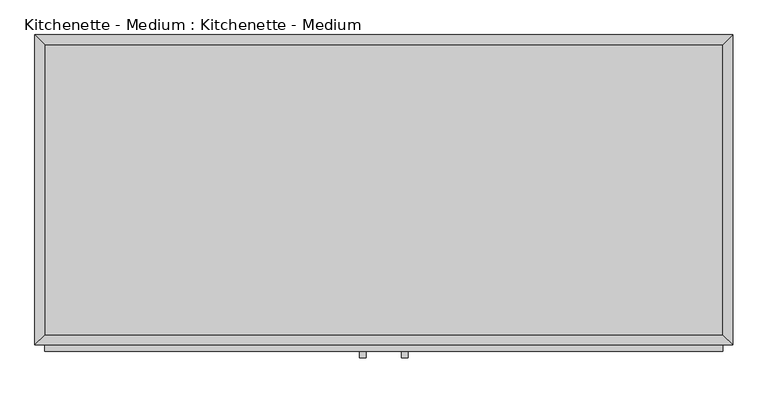
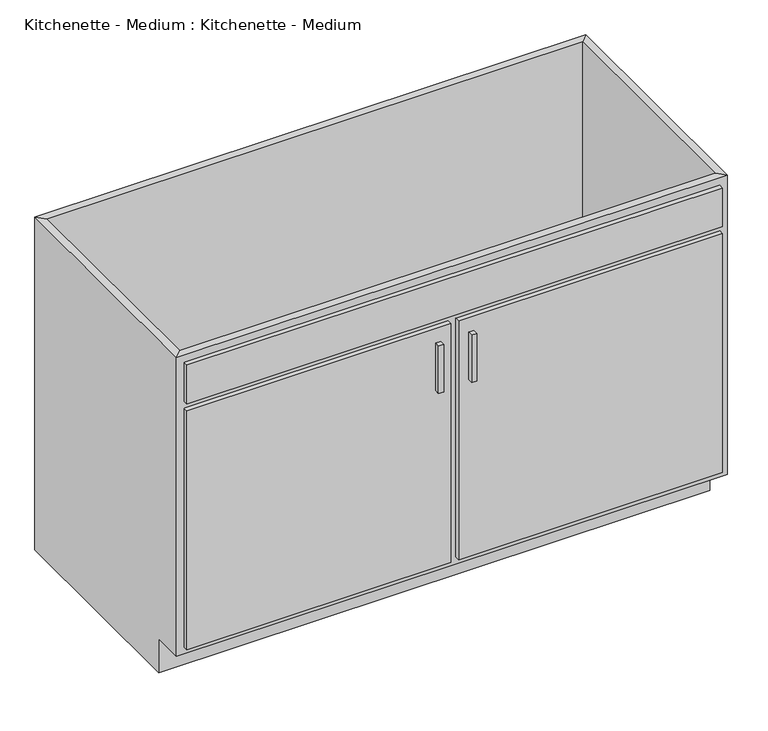
"""IFC4 building model written with IfcOpenShell, lengths in millimetres: proxy geometry, Kitchenette - Medium : Kitchenette - Medium."""

from ifc_helpers import new_model, si_unit, frame, origin, place, context, project, spatial, polyline, outline, extrude, faceted_brep, source, transform, mapped, element, save


def kitchenette_medium_kitchenette_medium_844211aa(model_context):
    return source(origin(), model_context, "Body", "SolidModel", [
        faceted_brep([(685.4877049, -590.55, 876.3), (685.4877049, -590.55, 88.9), (-648.0122951, -590.55, 88.9), (-648.0122951, -590.55, 876.3), (-667.0622951, -609.6, 876.3), (704.5377049, -609.6, 876.3), (-667.0622951, -609.6, 88.9), (704.5377049, -609.6, 88.9), (-648.0122951, -533.4, 88.9), (-648.0122951, -19.05, 88.9), (-648.0122951, -19.05, 876.3), (-667.0622951, 0.0, 876.3), (-667.0622951, 0.0, 0.0), (-667.0622951, -533.4, 0.0), (-667.0622951, -533.4, 88.9), (685.4877049, -19.05, 88.9), (685.4877049, -19.05, 876.3), (704.5377049, 0.0, 876.3), (704.5377049, 0.0, 0.0), (685.4877049, -533.4, 88.9), (704.5377049, -533.4, 88.9), (704.5377049, -533.4, 0.0)], [[[0, 1, 2, 3]], [[0, 3, 4, 5]], [[5, 4, 6, 7]], [[2, 1, 7, 6]], [[3, 2, 8, 9, 10]], [[4, 3, 10, 11]], [[6, 4, 11, 12, 13, 14]], [[2, 6, 14, 8]], [[10, 9, 15, 16]], [[11, 10, 16, 17]], [[12, 11, 17, 18]], [[1, 0, 16, 15, 19]], [[0, 5, 17, 16]], [[5, 7, 20, 21, 18, 17]], [[7, 1, 19, 20]], [[8, 19, 15, 9]], [[18, 21, 13, 12]], [[13, 21, 20, 19, 8, 14]]]),
        extrude(outline(polyline([(-16.1872951, -635.0), (-28.8872951, -635.0), (-28.8872951, -622.3), (-16.1872951, -622.3), (-16.1872951, -635.0)])), frame((0.0, 0.0, 573.769895), z_axis=(0.0, 0.0, 1.0), x_axis=(1.0, 0.0, 0.0)), (0.0, 0.0, 1.0), 124.730105),
        extrude(outline(polyline([(66.3627049, -635.0), (53.6627049, -635.0), (53.6627049, -622.3), (66.3627049, -622.3), (66.3627049, -635.0)])), frame((0.0, 0.0, 573.769895), z_axis=(0.0, 0.0, 1.0), x_axis=(1.0, 0.0, 0.0)), (0.0, 0.0, 1.0), 124.730105),
        extrude(outline(polyline([(685.4877049, -19.05), (685.4877049, -590.55), (-648.0122951, -590.55), (-648.0122951, -19.05), (685.4877049, -19.05)])), frame((0.0, 0.0, 88.9), z_axis=(0.0, 0.0, 1.0), x_axis=(1.0, 0.0, 0.0)), (0.0, 0.0, 1.0), 19.05),
        extrude(outline(polyline([(9.2127049, -622.3), (-648.0122951, -622.3), (-648.0122951, -609.6), (9.2127049, -609.6), (9.2127049, -622.3)])), frame((0.0, 0.0, 107.95), z_axis=(0.0, 0.0, 1.0), x_axis=(1.0, 0.0, 0.0)), (0.0, 0.0, 1.0), 628.65),
        extrude(outline(polyline([(685.4877049, -622.3), (28.2627049, -622.3), (28.2627049, -609.6), (685.4877049, -609.6), (685.4877049, -622.3)])), frame((0.0, 0.0, 107.95), z_axis=(0.0, 0.0, 1.0), x_axis=(1.0, 0.0, 0.0)), (0.0, 0.0, 1.0), 628.65),
        extrude(outline(polyline([(685.4877049, -622.3), (-648.0122951, -622.3), (-648.0122951, -609.6), (685.4877049, -609.6), (685.4877049, -622.3)])), frame((0.0, 0.0, 755.65), z_axis=(0.0, 0.0, 1.0), x_axis=(1.0, 0.0, 0.0)), (0.0, 0.0, 1.0), 101.6),
    ])


if __name__ == "__main__":
    model = new_model("IFC4")
    model_context = context("Model", 3, world=origin())
    ifc_project = project(units=[si_unit("LENGTHUNIT", "METRE", prefix="MILLI")], contexts=[model_context])
    site = spatial("IfcSite", under=ifc_project)
    building = spatial("IfcBuilding", under=site)
    placement = place(None, origin())
    kitchenette_medium_kitchenette_medium_shape = kitchenette_medium_kitchenette_medium_844211aa(model_context)
    element("IfcBuildingElementProxy", 1, Name="Kitchenette - Medium : Kitchenette - Medium", ObjectType="Kitchenette - Medium : Kitchenette - Medium", at=placement, inside=building, context=model_context, shape_type="MappedRepresentation", body=[
        mapped(kitchenette_medium_kitchenette_medium_shape, transform((0.0, 0.0, 0.0), x_axis=(1.0, 0.0, 0.0), y_axis=(0.0, 1.0, 0.0), z_axis=(0.0, 0.0, 1.0))),
    ])
    save(model, "model.ifc")

# Revit data of these elements
# Type "Kitchenette - Medium : Kitchenette - Medium"
#   Assembly Code = "E1090400"
#   Counter Length = 6' - 6"
#   Cabinet Width = 4' - 6"
#   Cabinet Height = 2' - 10 1/2"
#   Cabinet Depth = 2' - 0"
#   Toe Depth = 0' - 3"
#   Toe Height = 0' - 3 1/2"
#   Cabinet Material = Cabinets
#   Door/Drawer Material = Cabinets
#   Handle Material = Cabinets - Handles
#   Default Elevation = 0
# Element 1 (IfcBuildingElementProxy, "Kitchenette - Medium : Kitchenette - Medium")
#   Materials on its faces: "Cabinets", "Cabinets - Handles"
# Materials
#   "Cabinets": colour RGB 249 249 249, transparency 0
#   "Cabinets - Handles": class "Metal", colour RGB 57 57 57, transparency 0
